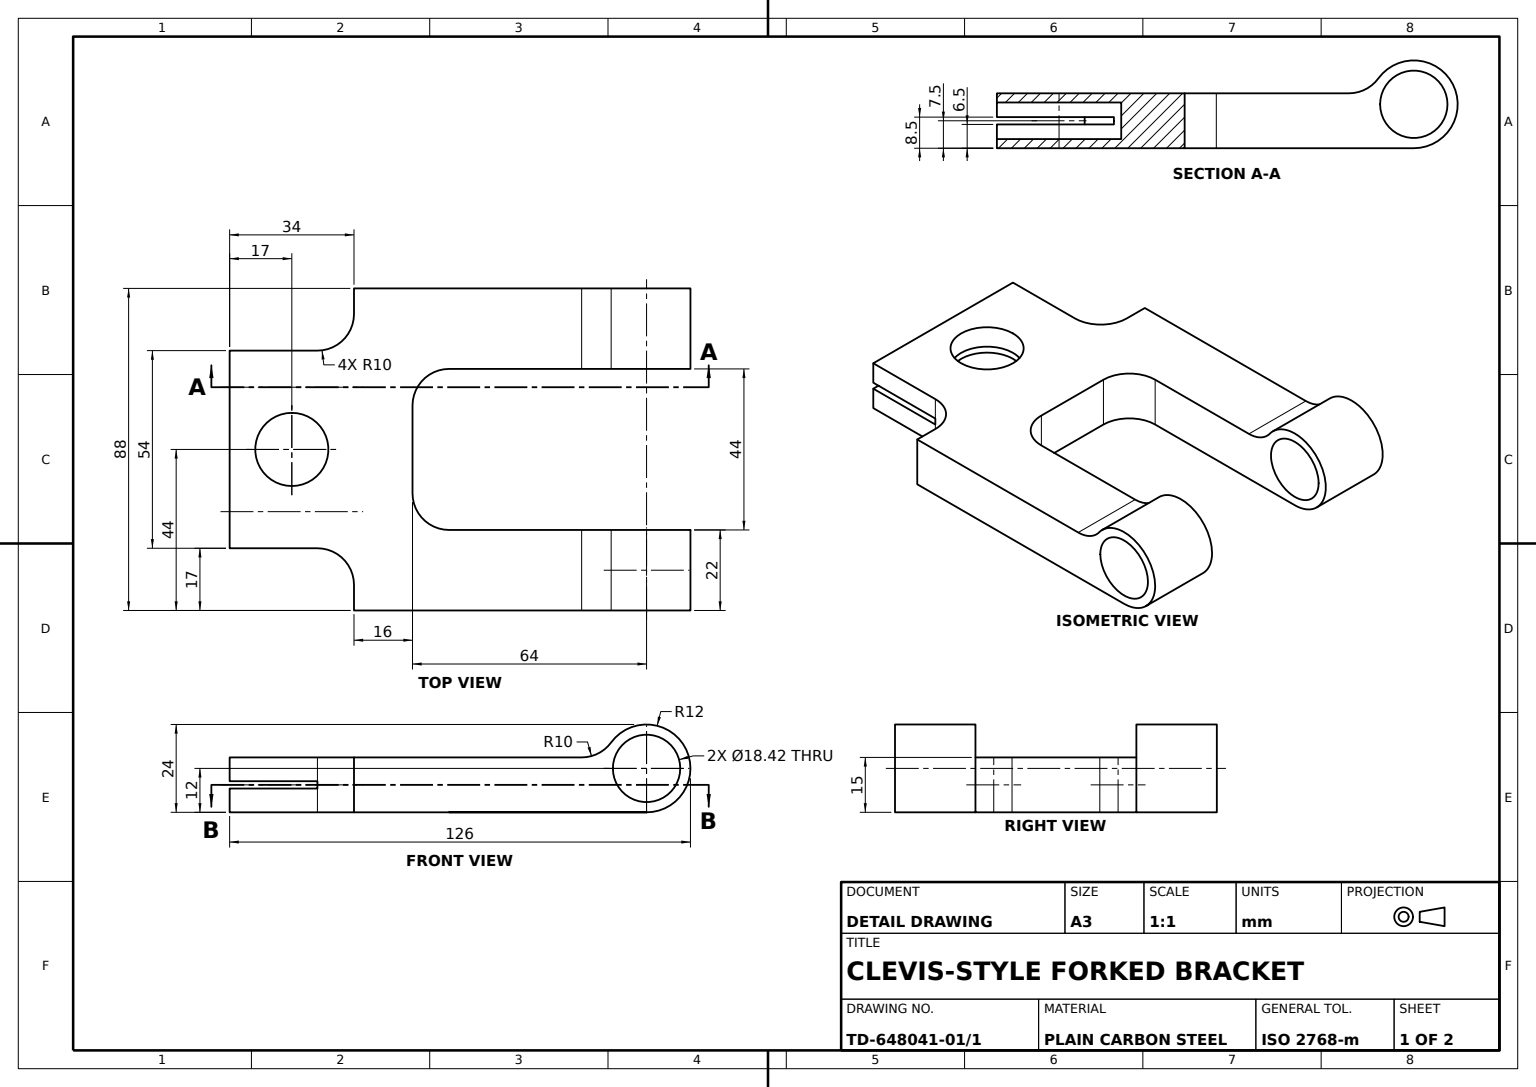
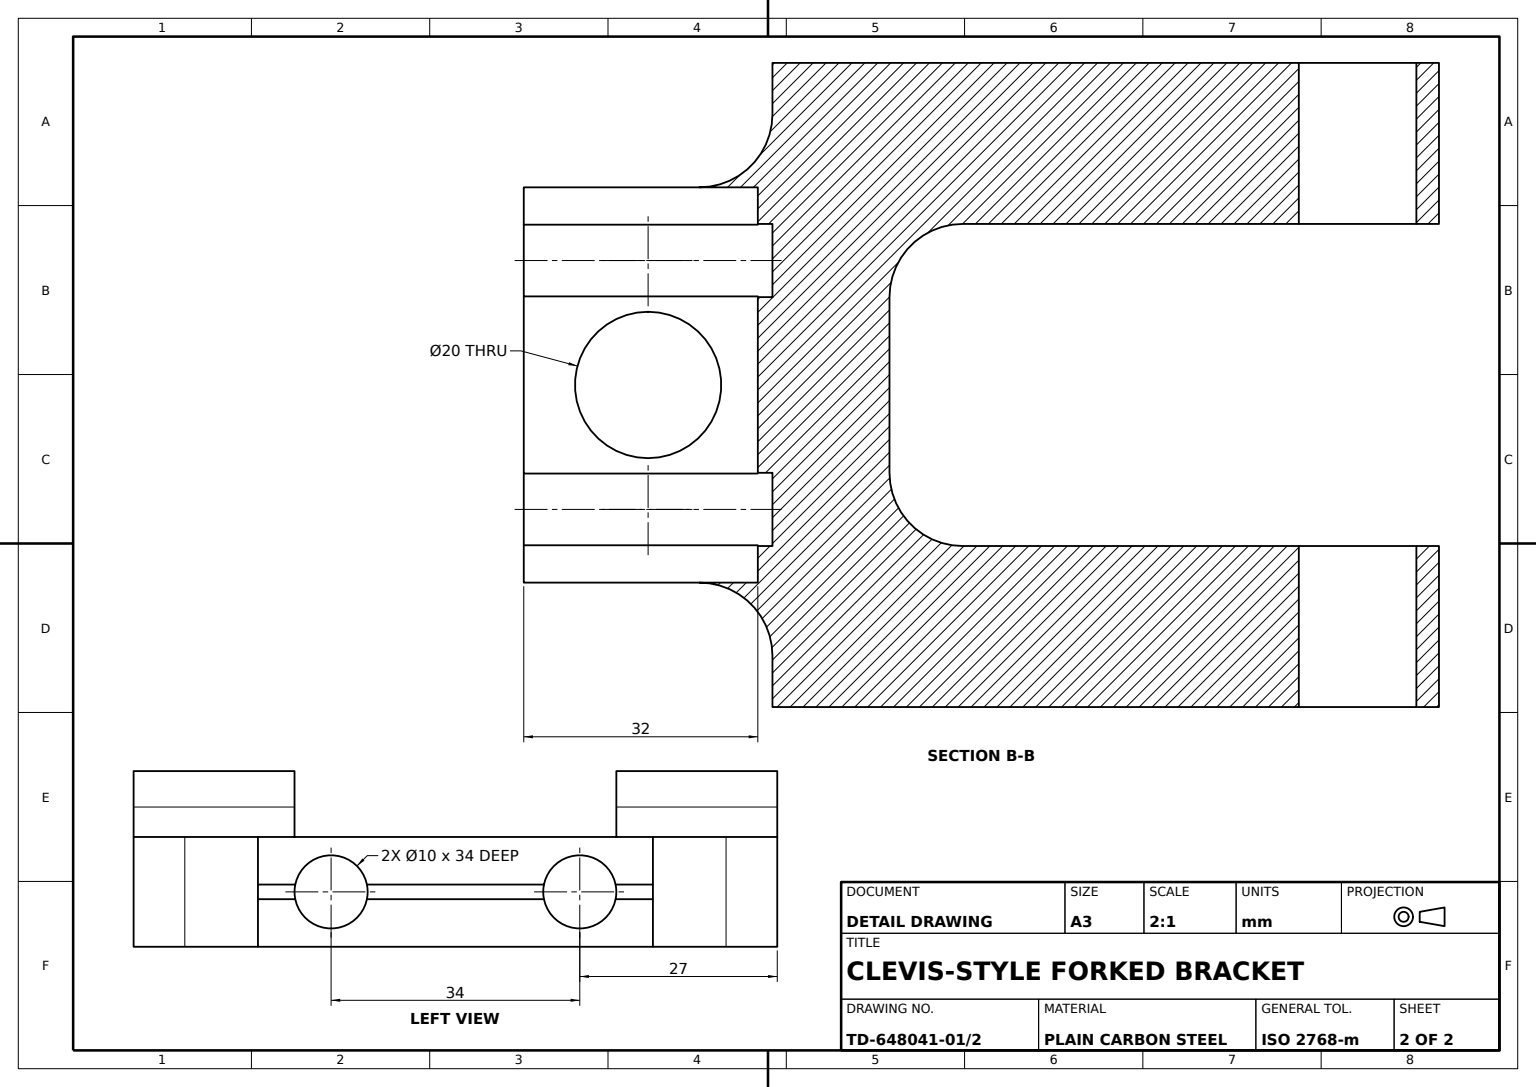
from build123d import *

# Parameters (mm, degrees)
BASE_PLATE_SKETCH_R     = 10
BASE_PLATE_DEPTH        = 7.5
KNUCKLE_A_SKETCH_R      = 12
KNUCKLE_A_SKETCH_R_2    = 9
KNUCKLE_A_DEPTH         = 22
KNUCKLE_A_BORE_SKETCH_R = 9.21075175
KNUCKLE_A_BORE_DEPTH    = 22
KNUCKLE_A_BLEND_R10_R   = 10
KNUCKLE_START           = -22
KNUCKLE_B_SKETCH_R      = 12
KNUCKLE_B_SKETCH_R_2    = 9.21075175
KNUCKLE_B_DEPTH         = 22
KNUCKLE_B_BORE_SKETCH_R = 9.21075175
KNUCKLE_B_BORE_DEPTH    = 22
KNUCKLE_B_BLEND_R10_R   = 10
GROOVE_CUT_SKETCH_W     = 54
GROOVE_CUT_SKETCH_H     = 2
GROOVE_CUT_DEPTH        = 32
HOLE_CUT_SKETCH_R       = 5
HOLE_CUT_DEPTH          = 34


with BuildPart() as part:
    # Base Plate Sketch → Base Plate (new, symmetric)
    with BuildSketch(Plane(origin=(0, 0, 0), x_dir=(1, 0, 0), z_dir=(0, 1, 0))):
        with BuildLine():
            Line((0, 44), (0, 22))
            Line((0, 22), (-54, 22))
            ThreePointArc((-54, 22), (-61.071067812, 19.071067812), (-64, 12))
            Line((-64, 12), (-64, -12))
            ThreePointArc((-64, -12), (-61.071067812, -19.071067812), (-54, -22))
            Line((-54, -22), (0, -22))
            Line((0, -22), (0, -44))
            Line((0, -44), (-64, -44))
            Line((-64, -44), (-80, -44))
            Line((-80, -44), (-80, -37))
            ThreePointArc((-80, -37), (-82.928932188, -29.928932188), (-90, -27))
            Line((-90, -27), (-114, -27))
            Line((-114, -27), (-114, 27))
            Line((-114, 27), (-90, 27))
            ThreePointArc((-90, 27), (-82.928932188, 29.928932188), (-80, 37))
            Line((-80, 37), (-80, 44))
            Line((-80, 44), (-64, 44))
            Line((-64, 44), (0, 44))
        make_face()
        with Locations(Location((-97, 0, 0), (0, 0, 270))):
            Circle(BASE_PLATE_SKETCH_R, mode=Mode.SUBTRACT)
    extrude(amount=BASE_PLATE_DEPTH, both=True)

    # Knuckle A Sketch → Knuckle A (add)
    with BuildSketch(Plane.XY.offset(44)):
        with Locations((0, 4.5)):
            Circle(KNUCKLE_A_SKETCH_R)
        with Locations((0, 4.5)):
            Circle(KNUCKLE_A_SKETCH_R_2, mode=Mode.SUBTRACT)
    extrude(amount=-KNUCKLE_A_DEPTH)

    # Knuckle A Bore Sketch → Knuckle A Bore (cut)
    with BuildSketch(Plane.XY.offset(44)):
        with Locations((0, 4.5)):
            Circle(KNUCKLE_A_BORE_SKETCH_R)
    extrude(amount=-KNUCKLE_A_BORE_DEPTH, mode=Mode.SUBTRACT)

    # Knuckle A Blend R10
    knuckle_a_blend_r10_edges = [part.edges().sort_by_distance(p)[0] for p in [
        (-11.618950039, 7.5, 33),
    ]]
    fillet(knuckle_a_blend_r10_edges, radius=KNUCKLE_A_BLEND_R10_R)

    # Knuckle B Sketch → Knuckle B (add)
    with BuildSketch(Plane(origin=(0, 0, -44), x_dir=(-1, 0, 0), z_dir=(0, 0, -1)).offset(KNUCKLE_START)):
        with Locations((0, 4.5)):
            Circle(KNUCKLE_B_SKETCH_R)
        with Locations(Location((0, 4.5, 0), (0, 0, 180))):
            Circle(KNUCKLE_B_SKETCH_R_2, mode=Mode.SUBTRACT)
    extrude(amount=KNUCKLE_B_DEPTH)

    # Knuckle B Bore Sketch → Knuckle B Bore (cut)
    with BuildSketch(Plane(origin=(0, 0, -44), x_dir=(-1, 0, 0), z_dir=(0, 0, -1)).offset(KNUCKLE_START)):
        with Locations(Location((0, 4.5, 0), (0, 0, 180))):
            Circle(KNUCKLE_B_BORE_SKETCH_R)
    extrude(amount=KNUCKLE_B_BORE_DEPTH, mode=Mode.SUBTRACT)

    # Knuckle B Blend R10
    knuckle_b_blend_r10_edges = [part.edges().sort_by_distance(p)[0] for p in [
        (-11.618950039, 7.5, -33),
    ]]
    fillet(knuckle_b_blend_r10_edges, radius=KNUCKLE_B_BLEND_R10_R)

    # Groove Cut Sketch → Groove Cut (cut)
    with BuildSketch(Plane.ZY.offset(114)):
        Rectangle(GROOVE_CUT_SKETCH_W, GROOVE_CUT_SKETCH_H)
    extrude(amount=-GROOVE_CUT_DEPTH, mode=Mode.SUBTRACT)

    # Hole Cut Sketch → Hole Cut (cut)
    with BuildSketch(Plane.ZY.offset(114)):
        with Locations((-17, 0)):
            Circle(HOLE_CUT_SKETCH_R)
        with Locations((17, 0)):
            Circle(HOLE_CUT_SKETCH_R)
    extrude(amount=-HOLE_CUT_DEPTH, mode=Mode.SUBTRACT)


solid = part.part
